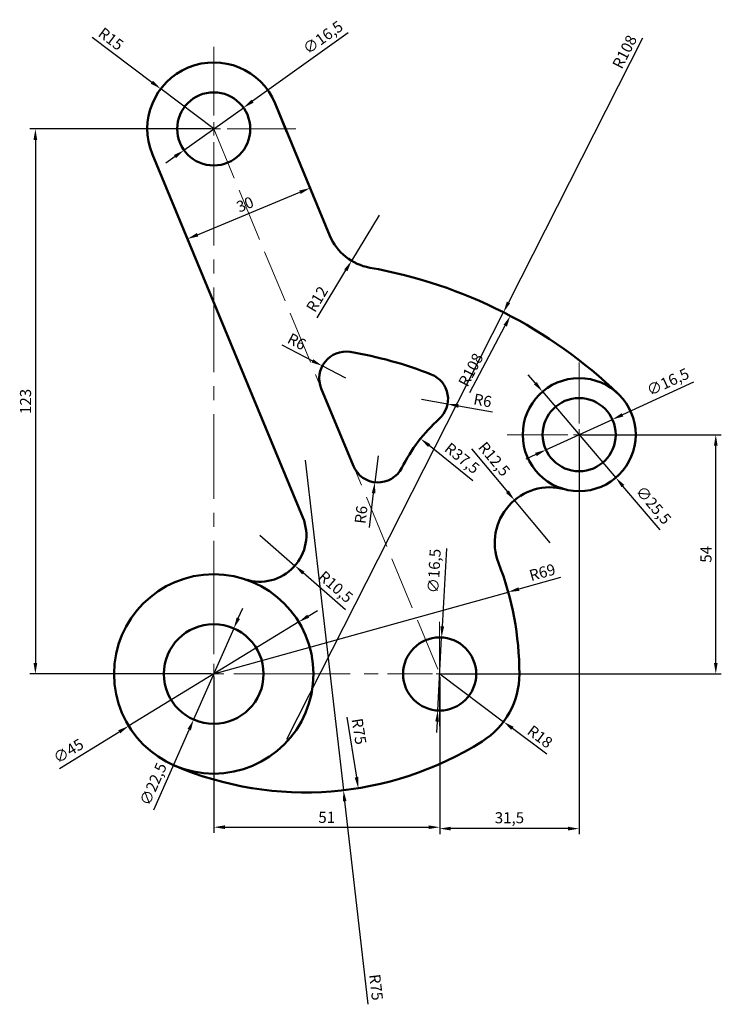
# Model space of a CAD drawing. Units: millimetres. Extents: x 2645 to 2804, y 1499 to 1721.
import ezdxf

# ---------------------------------------------------------------- set-up
doc = ezdxf.new("R2010")
doc.units = ezdxf.units.MM
doc.linetypes.add('ACAD_ISO02W100', pattern=[15, 12, -3])
doc.linetypes.add('CENTER2', pattern=[28.575, 19.05, -3.175, 3.175, -3.175])
for name, color, linetype, lineweight in [('M-CNTR', 4, 'CENTER2', 18), ('M-CONS', 8, 'ACAD_ISO02W100', 18), ('M-DIMS', 2, 'Continuous', 25), ('M-OUTL', 7, 'Continuous', 50)]:
    doc.layers.add(name, color=color, linetype=linetype, lineweight=lineweight)
doc.styles.get("Standard").update_dxf_attribs({"font": 'arial.ttf'})
doc.dimstyles.new('ISO-25', dxfattribs={"dimtxt": 2.5, "dimasz": 2.5, "dimexe": 1.25, "dimexo": 0.625, "dimtad": 1, "dimtxsty": 'Standard', "dimcen": 2.5, "dimadec": 0, "dimazin": 0, "dimtfac": 1, "dimtmove": 0, "dimatfit": 3, "dimfxl": 1, "dimarcsym": 0})

# ---------------------------------------------------------------- blocks, each defined once
blk = doc.blocks.new('*U1')
at = {"layer": 'M-CNTR', "color": 0, "transparency": 16777216}
for p, q in [((0, 4.5), (0, 26)), ((-26, 0), (-4.5, 0)), ((4.5, 0), (26, 0)), ((0, -26), (0, -4.5))]:
    blk.add_line(p, q, dxfattribs=at)
at = {"layer": 'M-CNTR', "color": 0, "linetype": 'Continuous', "transparency": 16777216}
for p, q in [((0, -2.25), (0, 2.25)), ((-2.25, 0), (2.25, 0))]:
    blk.add_line(p, q, dxfattribs=at)
blk = doc.blocks.new('*U2')
at = {"layer": 'M-CNTR', "color": 0, "transparency": 16777216}
for p, q in [((0, 2.55), (0, 16.25)), ((-16.25, 0), (-2.55, 0)), ((2.55, 0), (16.25, 0)), ((0, -16.25), (0, -2.55))]:
    blk.add_line(p, q, dxfattribs=at)
at = {"layer": 'M-CNTR', "color": 0, "linetype": 'Continuous', "transparency": 16777216}
for p, q in [((-1.275, 0), (1.275, 0)), ((0, -1.275), (0, 1.275))]:
    blk.add_line(p, q, dxfattribs=at)
blk = doc.blocks.new('*U3')
at = {"layer": 'M-CNTR', "color": 0, "transparency": 16777216}
for p, q in [((0, 3), (0, 18.5)), ((-18.5, 0), (-3, 0)), ((3, 0), (18.5, 0)), ((0, -18.5), (0, -3))]:
    blk.add_line(p, q, dxfattribs=at)
at = {"layer": 'M-CNTR', "color": 0, "linetype": 'Continuous', "transparency": 16777216}
for p, q in [((-1.5, 0), (1.5, 0)), ((0, -1.5), (0, 1.5))]:
    blk.add_line(p, q, dxfattribs=at)
blk = doc.blocks.new('*U4')
at = {"layer": 'M-CNTR', "color": 0, "transparency": 16777216}
for p, q in [((0, 1.65), (0, 11.75)), ((-11.75, 0), (-1.65, 0)), ((1.65, 0), (11.75, 0)), ((0, -11.75), (0, -1.65))]:
    blk.add_line(p, q, dxfattribs=at)
at = {"layer": 'M-CNTR', "color": 0, "linetype": 'Continuous', "transparency": 16777216}
for p, q in [((-0.825, 0), (0.825, 0)), ((0, -0.825), (0, 0.825))]:
    blk.add_line(p, q, dxfattribs=at)
blk = doc.blocks.new('*U5')
at = {"layer": 'M-CNTR', "color": 0, "transparency": 16777216}
blk.add_line((0, 52), (0, -52), dxfattribs=at)
blk = doc.blocks.new('*U6')
at = {"layer": 'M-CNTR', "color": 0, "transparency": 16777216}
blk.add_line((-18.025, 0), (18.025, 0), dxfattribs=at)
blk = doc.blocks.new('*D7')
at = {"layer": 'Defpoints', "color": 0, "transparency": 16777216}
for p in [(2689.12, 1696.37), (2648.85, 1573.37), (2689.12, 1573.37)]:
    blk.add_point(p, dxfattribs=at)
at = {"layer": 'M-DIMS', "color": 0, "lineweight": -2, "transparency": 16777216}
for p, q in [((2688.49, 1696.37), (2647.6, 1696.37)), ((2648.85, 1693.87), (2648.85, 1575.87)), ((2688.49, 1573.37), (2647.6, 1573.37))]:
    blk.add_line(p, q, dxfattribs=at)
at = {"layer": 'M-DIMS', "color": 0, "transparency": 16777216}
for points in [[(2648.43, 1693.87), (2649.27, 1693.87), (2648.85, 1696.37)], [(2648.43, 1575.87), (2649.27, 1575.87), (2648.85, 1573.37)]]:
    blk.add_solid(points, dxfattribs=at)
at = {"layer": 'M-DIMS', "color": 0, "transparency": 16777216, "insert": (2646.95, 1634.87), "char_height": 2.5, "attachment_point": 5, "rotation": 90}
blk.add_mtext('123', dxfattribs=at)
blk = doc.blocks.new('*D8')
at = {"layer": 'Defpoints', "color": 0, "transparency": 16777216}
for p in [(2689.12, 1573.37), (2740.12, 1573.37), (2740.12, 1538.79)]:
    blk.add_point(p, dxfattribs=at)
at = {"layer": 'M-DIMS', "color": 0, "lineweight": -2, "transparency": 16777216}
for p, q in [((2689.12, 1572.75), (2689.12, 1537.54)), ((2740.12, 1572.75), (2740.12, 1537.54)), ((2691.62, 1538.79), (2737.62, 1538.79))]:
    blk.add_line(p, q, dxfattribs=at)
at = {"layer": 'M-DIMS', "color": 0, "transparency": 16777216}
for points in [[(2691.62, 1539.21), (2691.62, 1538.38), (2689.12, 1538.79)], [(2737.62, 1539.21), (2737.62, 1538.38), (2740.12, 1538.79)]]:
    blk.add_solid(points, dxfattribs=at)
at = {"layer": 'M-DIMS', "color": 0, "transparency": 16777216, "insert": (2714.62, 1540.69), "char_height": 2.5, "attachment_point": 5}
blk.add_mtext('51', dxfattribs=at)
blk = doc.blocks.new('*D9')
at = {"layer": 'Defpoints', "color": 0, "transparency": 16777216}
for p in [(2771.62, 1627.37), (2740.12, 1572.81), (2740.12, 1538.47)]:
    blk.add_point(p, dxfattribs=at)
at = {"layer": 'M-DIMS', "color": 0, "lineweight": -2, "transparency": 16777216}
for p, q in [((2771.62, 1626.75), (2771.62, 1537.22)), ((2740.12, 1572.19), (2740.12, 1537.22)), ((2769.12, 1538.47), (2742.62, 1538.47))]:
    blk.add_line(p, q, dxfattribs=at)
at = {"layer": 'M-DIMS', "color": 0, "transparency": 16777216}
for points in [[(2742.62, 1538.89), (2742.62, 1538.06), (2740.12, 1538.47)], [(2769.12, 1538.89), (2769.12, 1538.06), (2771.62, 1538.47)]]:
    blk.add_solid(points, dxfattribs=at)
at = {"layer": 'M-DIMS', "color": 0, "transparency": 16777216, "insert": (2755.87, 1540.6), "char_height": 2.5, "attachment_point": 5}
blk.add_mtext('31,5', dxfattribs=at)
blk = doc.blocks.new('*D10')
at = {"layer": 'Defpoints', "color": 0, "transparency": 16777216}
for p in [(2771.62, 1627.37), (2802.45, 1627.37), (2740.12, 1573.37)]:
    blk.add_point(p, dxfattribs=at)
at = {"layer": 'M-DIMS', "color": 0, "lineweight": -2, "transparency": 16777216}
for p, q in [((2772.24, 1627.37), (2803.7, 1627.37)), ((2802.45, 1575.87), (2802.45, 1624.87)), ((2740.74, 1573.37), (2803.7, 1573.37))]:
    blk.add_line(p, q, dxfattribs=at)
at = {"layer": 'M-DIMS', "color": 0, "transparency": 16777216}
for points in [[(2802.03, 1624.87), (2802.87, 1624.87), (2802.45, 1627.37)], [(2802.03, 1575.87), (2802.87, 1575.87), (2802.45, 1573.37)]]:
    blk.add_solid(points, dxfattribs=at)
at = {"layer": 'M-DIMS', "color": 0, "transparency": 16777216, "insert": (2800.56, 1600.37), "char_height": 2.5, "attachment_point": 5, "rotation": 90}
blk.add_mtext('54', dxfattribs=at)
blk = doc.blocks.new('*D11')
at = {"layer": 'Defpoints', "color": 0, "transparency": 16777216}
for p in [(2708.31, 1585.11), (2669.92, 1561.63)]:
    blk.add_point(p, dxfattribs=at)
at = {"layer": 'M-DIMS', "color": 0, "lineweight": -2, "transparency": 16777216}
for p, q in [((2710.44, 1586.42), (2712.57, 1587.72)), ((2708.31, 1585.11), (2669.92, 1561.63)), ((2654.28, 1552.06), (2667.79, 1560.33))]:
    blk.add_line(p, q, dxfattribs=at)
at = {"layer": 'M-DIMS', "color": 0, "transparency": 16777216}
for points in [[(2710.22, 1586.77), (2710.66, 1586.06), (2708.31, 1585.11)], [(2667.57, 1560.68), (2668.01, 1559.97), (2669.92, 1561.63)]]:
    blk.add_solid(points, dxfattribs=at)
at = {"layer": 'M-DIMS', "color": 0, "transparency": 16777216, "insert": (2656.48, 1555.72), "char_height": 2.5, "attachment_point": 5, "rotation": 31.4542}
blk.add_mtext('∅45', dxfattribs=at)
blk = doc.blocks.new('*D12')
at = {"layer": 'Defpoints', "color": 0, "transparency": 16777216}
for p in [(2693.65, 1583.66), (2684.58, 1563.08)]:
    blk.add_point(p, dxfattribs=at)
at = {"layer": 'M-DIMS', "color": 0, "lineweight": -2, "transparency": 16777216}
for p, q in [((2694.66, 1585.95), (2695.67, 1588.24)), ((2693.65, 1583.66), (2684.58, 1563.08)), ((2675.6, 1542.71), (2683.57, 1560.79))]:
    blk.add_line(p, q, dxfattribs=at)
at = {"layer": 'M-DIMS', "color": 0, "transparency": 16777216}
for points in [[(2694.28, 1586.12), (2695.04, 1585.78), (2693.65, 1583.66)], [(2683.19, 1560.96), (2683.95, 1560.62), (2684.58, 1563.08)]]:
    blk.add_solid(points, dxfattribs=at)
at = {"layer": 'M-DIMS', "color": 0, "transparency": 16777216, "insert": (2675.73, 1548.39), "char_height": 2.5, "attachment_point": 5, "rotation": 66.2096}
blk.add_mtext('∅22,5', dxfattribs=at)
blk = doc.blocks.new('*D13')
at = {"layer": 'Defpoints', "color": 0, "transparency": 16777216}
for p in [(2763.35, 1637.08), (2779.88, 1617.66)]:
    blk.add_point(p, dxfattribs=at)
at = {"layer": 'M-DIMS', "color": 0, "lineweight": -2, "transparency": 16777216}
for p, q in [((2761.73, 1638.98), (2760.11, 1640.88)), ((2763.35, 1637.08), (2779.88, 1617.66)), ((2789.92, 1605.88), (2781.5, 1615.76))]:
    blk.add_line(p, q, dxfattribs=at)
at = {"layer": 'M-DIMS', "color": 0, "transparency": 16777216}
for points in [[(2762.04, 1639.25), (2761.41, 1638.71), (2763.35, 1637.08)], [(2781.82, 1616.03), (2781.19, 1615.49), (2779.88, 1617.66)]]:
    blk.add_solid(points, dxfattribs=at)
at = {"layer": 'M-DIMS', "color": 0, "transparency": 16777216, "insert": (2788.17, 1611.27), "char_height": 2.5, "attachment_point": 5, "rotation": 310.4214}
blk.add_mtext('∅25,5', dxfattribs=at)
blk = doc.blocks.new('*D14')
at = {"layer": 'Defpoints', "color": 0, "transparency": 16777216}
for p in [(2695.83, 1701.16), (2682.4, 1691.58)]:
    blk.add_point(p, dxfattribs=at)
at = {"layer": 'M-DIMS', "color": 0, "lineweight": -2, "transparency": 16777216}
for p, q in [((2719.47, 1718.04), (2697.86, 1702.62)), ((2682.4, 1691.58), (2695.83, 1701.16)), ((2680.37, 1690.12), (2678.33, 1688.67))]:
    blk.add_line(p, q, dxfattribs=at)
at = {"layer": 'M-DIMS', "color": 0, "transparency": 16777216}
for points in [[(2697.62, 1702.96), (2698.11, 1702.28), (2695.83, 1701.16)], [(2680.12, 1690.46), (2680.61, 1689.79), (2682.4, 1691.58)]]:
    blk.add_solid(points, dxfattribs=at)
at = {"layer": 'M-DIMS', "color": 0, "transparency": 16777216, "insert": (2713.95, 1716.76), "char_height": 2.5, "attachment_point": 5, "rotation": 35.5241}
blk.add_mtext('∅16,5', dxfattribs=at)
blk = doc.blocks.new('*D15')
at = {"layer": 'Defpoints', "color": 0, "transparency": 16777216}
for p in [(2779.12, 1630.81), (2764.11, 1623.94)]:
    blk.add_point(p, dxfattribs=at)
at = {"layer": 'M-DIMS', "color": 0, "lineweight": -2, "transparency": 16777216}
for p, q in [((2797.44, 1639.2), (2781.39, 1631.85)), ((2764.11, 1623.94), (2779.12, 1630.81)), ((2761.84, 1622.89), (2759.57, 1621.85))]:
    blk.add_line(p, q, dxfattribs=at)
at = {"layer": 'M-DIMS', "color": 0, "transparency": 16777216}
for points in [[(2781.22, 1632.23), (2781.56, 1631.47), (2779.12, 1630.81)], [(2761.67, 1623.27), (2762.02, 1622.52), (2764.11, 1623.94)]]:
    blk.add_solid(points, dxfattribs=at)
at = {"layer": 'M-DIMS', "color": 0, "transparency": 16777216, "insert": (2791.77, 1638.99), "char_height": 2.5, "attachment_point": 5, "rotation": 24.6069}
blk.add_mtext('∅16,5', dxfattribs=at)
blk = doc.blocks.new('*D16')
at = {"layer": 'Defpoints', "color": 0, "transparency": 16777216}
for p in [(2740.56, 1581.61), (2739.67, 1565.13)]:
    blk.add_point(p, dxfattribs=at)
at = {"layer": 'M-DIMS', "color": 0, "lineweight": -2, "transparency": 16777216}
for p, q in [((2741.64, 1601.71), (2740.69, 1584.11)), ((2739.67, 1565.13), (2740.56, 1581.61)), ((2739.54, 1562.64), (2739.41, 1560.14))]:
    blk.add_line(p, q, dxfattribs=at)
at = {"layer": 'M-DIMS', "color": 0, "transparency": 16777216}
for points in [[(2740.28, 1584.13), (2741.11, 1584.08), (2740.56, 1581.61)], [(2739.12, 1562.66), (2739.96, 1562.61), (2739.67, 1565.13)]]:
    blk.add_solid(points, dxfattribs=at)
at = {"layer": 'M-DIMS', "color": 0, "transparency": 16777216, "insert": (2739.19, 1596.59), "char_height": 2.5, "attachment_point": 5, "rotation": 86.9302}
blk.add_mtext('∅16,5', dxfattribs=at)
blk = doc.blocks.new('*D17')
at = {"layer": 'Defpoints', "color": 0, "transparency": 16777216}
for p in [(2677.14, 1705.41), (2689.12, 1696.37)]:
    blk.add_point(p, dxfattribs=at)
at = {"layer": 'M-DIMS', "color": 0, "lineweight": -2, "transparency": 16777216}
for p, q in [((2661.68, 1717.08), (2675.15, 1706.91)), ((2689.12, 1696.37), (2677.14, 1705.41))]:
    blk.add_line(p, q, dxfattribs=at)
at = {"layer": 'M-DIMS', "color": 0, "transparency": 16777216}
blk.add_solid([(2675.4, 1707.25), (2674.9, 1706.58), (2677.14, 1705.41)], dxfattribs=at)
at = {"layer": 'M-DIMS', "color": 0, "transparency": 16777216, "insert": (2665.72, 1716.42), "char_height": 2.5, "attachment_point": 5, "rotation": 322.951}
blk.add_mtext('R15', dxfattribs=at)
blk = doc.blocks.new('*D18')
at = {"layer": 'Defpoints', "color": 0, "transparency": 16777216}
for p in [(2726.43, 1676.87), (2720.23, 1666.6)]:
    blk.add_point(p, dxfattribs=at)
at = {"layer": 'M-DIMS', "color": 0, "lineweight": -2, "transparency": 16777216}
for p, q in [((2726.43, 1676.87), (2720.23, 1666.6)), ((2712.46, 1653.73), (2718.94, 1664.46))]:
    blk.add_line(p, q, dxfattribs=at)
at = {"layer": 'M-DIMS', "color": 0, "transparency": 16777216}
blk.add_solid([(2718.58, 1664.67), (2719.29, 1664.24), (2720.23, 1666.6)], dxfattribs=at)
at = {"layer": 'M-DIMS', "color": 0, "transparency": 16777216, "insert": (2712.71, 1657.79), "char_height": 2.5, "attachment_point": 5, "rotation": 58.8826}
blk.add_mtext('R12', dxfattribs=at)
blk = doc.blocks.new('*D19')
at = {"layer": 'Defpoints', "color": 0, "transparency": 16777216}
for p in [(2756.08, 1654.18), (2705.62, 1558.69)]:
    blk.add_point(p, dxfattribs=at)
at = {"layer": 'M-DIMS', "color": 0, "lineweight": -2, "transparency": 16777216}
blk.add_line((2746.95, 1636.91), (2754.91, 1651.97), dxfattribs=at)
at = {"layer": 'M-DIMS', "color": 0, "transparency": 16777216}
blk.add_solid([(2754.54, 1652.16), (2755.28, 1651.77), (2756.08, 1654.18)], dxfattribs=at)
at = {"layer": 'M-DIMS', "color": 0, "transparency": 16777216, "insert": (2747.42, 1641.85), "char_height": 2.5, "attachment_point": 5, "rotation": 62.146}
blk.add_mtext('R108', dxfattribs=at)
blk = doc.blocks.new('*D20')
at = {"layer": 'Defpoints', "color": 0, "transparency": 16777216}
for p in [(2757.02, 1612.58), (2765.04, 1602.99)]:
    blk.add_point(p, dxfattribs=at)
at = {"layer": 'M-DIMS', "color": 0, "lineweight": -2, "transparency": 16777216}
for p, q in [((2747.29, 1624.2), (2755.41, 1614.49)), ((2765.04, 1602.99), (2757.02, 1612.58))]:
    blk.add_line(p, q, dxfattribs=at)
at = {"layer": 'M-DIMS', "color": 0, "transparency": 16777216}
blk.add_solid([(2755.73, 1614.76), (2755.09, 1614.22), (2757.02, 1612.58)], dxfattribs=at)
at = {"layer": 'M-DIMS', "color": 0, "transparency": 16777216, "insert": (2752.18, 1621.67), "char_height": 2.5, "attachment_point": 5, "rotation": 309.937}
blk.add_mtext('R12,5', dxfattribs=at)
blk = doc.blocks.new('*D21')
at = {"layer": 'Defpoints', "color": 0, "transparency": 16777216}
for p in [(2735.8, 1626.47), (2765.04, 1602.99)]:
    blk.add_point(p, dxfattribs=at)
at = {"layer": 'M-DIMS', "color": 0, "lineweight": -2, "transparency": 16777216}
blk.add_line((2747.62, 1616.98), (2737.75, 1624.9), dxfattribs=at)
at = {"layer": 'M-DIMS', "color": 0, "transparency": 16777216}
blk.add_solid([(2738.01, 1625.23), (2737.49, 1624.58), (2735.8, 1626.47)], dxfattribs=at)
at = {"layer": 'M-DIMS', "color": 0, "transparency": 16777216, "insert": (2744.99, 1621.82), "char_height": 2.5, "attachment_point": 5, "rotation": 321.2426}
blk.add_mtext('R37,5', dxfattribs=at)
blk = doc.blocks.new('*D22')
at = {"layer": 'Defpoints', "color": 0, "transparency": 16777216}
for p in [(2713.62, 1642.88), (2718.94, 1640.11)]:
    blk.add_point(p, dxfattribs=at)
at = {"layer": 'M-DIMS', "color": 0, "lineweight": -2, "transparency": 16777216}
for p, q in [((2704.5, 1647.62), (2711.4, 1644.03)), ((2718.94, 1640.11), (2713.62, 1642.88))]:
    blk.add_line(p, q, dxfattribs=at)
at = {"layer": 'M-DIMS', "color": 0, "transparency": 16777216}
blk.add_solid([(2711.59, 1644.4), (2711.21, 1643.66), (2713.62, 1642.88)], dxfattribs=at)
at = {"layer": 'M-DIMS', "color": 0, "transparency": 16777216, "insert": (2707.72, 1648.09), "char_height": 2.5, "attachment_point": 5, "rotation": 332.5021}
blk.add_mtext('R6', dxfattribs=at)
blk = doc.blocks.new('*D23')
at = {"layer": 'Defpoints', "color": 0, "transparency": 16777216}
for p in [(2736.01, 1635.39), (2741.91, 1634.3)]:
    blk.add_point(p, dxfattribs=at)
at = {"layer": 'M-DIMS', "color": 0, "lineweight": -2, "transparency": 16777216}
for p, q in [((2736.01, 1635.39), (2741.91, 1634.3)), ((2752.02, 1632.43), (2744.37, 1633.84))]:
    blk.add_line(p, q, dxfattribs=at)
at = {"layer": 'M-DIMS', "color": 0, "transparency": 16777216}
blk.add_solid([(2744.45, 1634.25), (2744.3, 1633.43), (2741.91, 1634.3)], dxfattribs=at)
at = {"layer": 'M-DIMS', "color": 0, "transparency": 16777216, "insert": (2749.77, 1634.78), "char_height": 2.5, "attachment_point": 5, "rotation": 349.5394}
blk.add_mtext('R6', dxfattribs=at)
blk = doc.blocks.new('*D24')
at = {"layer": 'Defpoints', "color": 0, "transparency": 16777216}
for p in [(2726.21, 1622.58), (2725.49, 1616.63)]:
    blk.add_point(p, dxfattribs=at)
at = {"layer": 'M-DIMS', "color": 0, "lineweight": -2, "transparency": 16777216}
for p, q in [((2726.21, 1622.58), (2725.49, 1616.63)), ((2724.26, 1606.42), (2725.19, 1614.15))]:
    blk.add_line(p, q, dxfattribs=at)
at = {"layer": 'M-DIMS', "color": 0, "transparency": 16777216}
blk.add_solid([(2724.78, 1614.2), (2725.6, 1614.1), (2725.49, 1616.63)], dxfattribs=at)
at = {"layer": 'M-DIMS', "color": 0, "transparency": 16777216, "insert": (2722.69, 1609.27), "char_height": 2.5, "attachment_point": 5, "rotation": 83.1412}
blk.add_mtext('R6', dxfattribs=at)
blk = doc.blocks.new('*D25')
at = {"layer": 'Defpoints', "color": 0, "transparency": 16777216}
for p in [(2709.78, 1621.63), (2721.74, 1547.59)]:
    blk.add_point(p, dxfattribs=at)
at = {"layer": 'M-DIMS', "color": 0, "lineweight": -2, "transparency": 16777216}
blk.add_line((2719.15, 1563.63), (2721.34, 1550.06), dxfattribs=at)
at = {"layer": 'M-DIMS', "color": 0, "transparency": 16777216}
blk.add_solid([(2721.75, 1550.12), (2720.93, 1549.99), (2721.74, 1547.59)], dxfattribs=at)
at = {"layer": 'M-DIMS', "color": 0, "transparency": 16777216, "insert": (2721.6, 1560.36), "char_height": 2.5, "attachment_point": 5, "rotation": 279.1695}
blk.add_mtext('R75', dxfattribs=at)
blk = doc.blocks.new('*D26')
at = {"layer": 'Defpoints', "color": 0, "transparency": 16777216}
for p in [(2699.53, 1604.69), (2707.45, 1597.8)]:
    blk.add_point(p, dxfattribs=at)
at = {"layer": 'M-DIMS', "color": 0, "lineweight": -2, "transparency": 16777216}
for p, q in [((2699.53, 1604.69), (2707.45, 1597.8)), ((2718.89, 1587.85), (2709.34, 1596.16))]:
    blk.add_line(p, q, dxfattribs=at)
at = {"layer": 'M-DIMS', "color": 0, "transparency": 16777216}
blk.add_solid([(2709.61, 1596.47), (2709.06, 1595.84), (2707.45, 1597.8)], dxfattribs=at)
at = {"layer": 'M-DIMS', "color": 0, "transparency": 16777216, "insert": (2716.45, 1592.79), "char_height": 2.5, "attachment_point": 5, "rotation": 319.0015}
blk.add_mtext('R10,5', dxfattribs=at)
blk = doc.blocks.new('*D27')
at = {"layer": 'Defpoints', "color": 0, "transparency": 16777216}
for p in [(2755.59, 1591.86), (2689.12, 1573.37)]:
    blk.add_point(p, dxfattribs=at)
at = {"layer": 'M-DIMS', "color": 0, "lineweight": -2, "transparency": 16777216}
for p, q in [((2767.37, 1595.14), (2758, 1592.53)), ((2689.12, 1573.37), (2755.59, 1591.86))]:
    blk.add_line(p, q, dxfattribs=at)
at = {"layer": 'M-DIMS', "color": 0, "transparency": 16777216}
blk.add_solid([(2757.89, 1592.93), (2758.11, 1592.13), (2755.59, 1591.86)], dxfattribs=at)
at = {"layer": 'M-DIMS', "color": 0, "transparency": 16777216, "insert": (2763.38, 1596), "char_height": 2.5, "attachment_point": 5, "rotation": 15.5436}
blk.add_mtext('R69', dxfattribs=at)
blk = doc.blocks.new('*D28')
at = {"layer": 'Defpoints', "color": 0, "transparency": 16777216}
for p in [(2740.12, 1573.37), (2754.54, 1562.6)]:
    blk.add_point(p, dxfattribs=at)
at = {"layer": 'M-DIMS', "color": 0, "lineweight": -2, "transparency": 16777216}
for p, q in [((2740.12, 1573.37), (2754.54, 1562.6)), ((2764.34, 1555.28), (2756.54, 1561.1))]:
    blk.add_line(p, q, dxfattribs=at)
at = {"layer": 'M-DIMS', "color": 0, "transparency": 16777216}
blk.add_solid([(2756.79, 1561.44), (2756.29, 1560.77), (2754.54, 1562.6)], dxfattribs=at)
at = {"layer": 'M-DIMS', "color": 0, "transparency": 16777216, "insert": (2762.58, 1558.97), "char_height": 2.5, "attachment_point": 5, "rotation": 323.2484}
blk.add_mtext('R18', dxfattribs=at)
blk = doc.blocks.new('*D29')
at = {"layer": 'Defpoints', "color": 0, "transparency": 16777216}
for p in [(2710.89, 1683.03), (2711.13, 1682.43), (2683.42, 1670.94)]:
    blk.add_point(p, dxfattribs=at)
at = {"layer": 'M-DIMS', "color": 0, "lineweight": -2, "transparency": 16777216}
for p, q in [((2710.89, 1683.01), (2710.41, 1684.19)), ((2685.48, 1672.5), (2708.58, 1682.07)), ((2683.18, 1671.52), (2682.69, 1672.69))]:
    blk.add_line(p, q, dxfattribs=at)
at = {"layer": 'M-DIMS', "color": 0, "transparency": 16777216}
for points in [[(2708.42, 1682.46), (2708.74, 1681.69), (2710.89, 1683.03)], [(2685.32, 1672.88), (2685.64, 1672.11), (2683.17, 1671.54)]]:
    blk.add_solid(points, dxfattribs=at)
at = {"layer": 'M-DIMS', "color": 0, "transparency": 16777216, "insert": (2696.3, 1679.04), "char_height": 2.5, "attachment_point": 5, "rotation": 22.5206}
blk.add_mtext('30', dxfattribs=at)
blk = doc.blocks.new('*D30')
at = {"layer": 'Defpoints', "color": 0, "transparency": 16777216}
for p in [(2754.52, 1654.98), (2705.62, 1558.69)]:
    blk.add_point(p, dxfattribs=at)
at = {"layer": 'M-DIMS', "color": 0, "lineweight": -2, "transparency": 16777216}
for p, q in [((2785.94, 1716.85), (2755.65, 1657.21)), ((2705.62, 1558.69), (2754.52, 1654.98))]:
    blk.add_line(p, q, dxfattribs=at)
at = {"layer": 'M-DIMS', "color": 0, "transparency": 16777216}
blk.add_solid([(2755.28, 1657.4), (2756.02, 1657.02), (2754.52, 1654.98)], dxfattribs=at)
at = {"layer": 'M-DIMS', "color": 0, "transparency": 16777216, "insert": (2782.16, 1713.62), "char_height": 2.5, "attachment_point": 5, "rotation": 63.0782}
blk.add_mtext('R108', dxfattribs=at)
blk = doc.blocks.new('*D31')
at = {"layer": 'Defpoints', "color": 0, "transparency": 16777216}
for p in [(2709.78, 1621.63), (2718.4, 1547.13)]:
    blk.add_point(p, dxfattribs=at)
at = {"layer": 'M-DIMS', "color": 0, "lineweight": -2, "transparency": 16777216}
for p, q in [((2709.78, 1621.63), (2718.4, 1547.13)), ((2723.98, 1498.83), (2718.69, 1544.64))]:
    blk.add_line(p, q, dxfattribs=at)
at = {"layer": 'M-DIMS', "color": 0, "transparency": 16777216}
blk.add_solid([(2719.1, 1544.69), (2718.27, 1544.6), (2718.4, 1547.13)], dxfattribs=at)
at = {"layer": 'M-DIMS', "color": 0, "transparency": 16777216, "insert": (2725.45, 1502.64), "char_height": 2.5, "attachment_point": 5, "rotation": 276.5954}
blk.add_mtext('R75', dxfattribs=at)

msp = doc.modelspace()

# ---------------------------------------------------------------- linework, layer by layer
at = {"layer": 'M-CONS'}
msp.add_line((2689.116, 1696.371), (2740.116, 1573.371), dxfattribs=at)
at = {"layer": 'M-OUTL'}
for p, q in [((2702.972, 1702.116), (2715.345, 1672.274)), ((2702.972, 1702.116), (2705.653, 1695.65)), ((2705.653, 1695.65), (2705.844, 1695.188)), ((2675.26, 1690.625), (2709.226, 1608.707)), ((2720.663, 1620.287), (2713.398, 1637.808))]:
    msp.add_line(p, q, dxfattribs=at)
for centre, radius in [((2689.116, 1696.371), 8.25), ((2771.616, 1627.371), 12.75), ((2771.616, 1627.371), 8.25), ((2689.116, 1573.371), 22.5), ((2689.116, 1573.371), 11.25), ((2740.116, 1573.371), 8.25)]:
    msp.add_circle(centre, radius, dxfattribs=at)
for centre, radius, start, end in [((2689.116, 1696.371), 15, 22.52057, 202.52057), ((2726.43, 1676.871), 12, 202.52057, 260.01375), ((2705.621, 1558.689), 108, 46.1429, 80.01375), ((2718.94, 1640.106), 6, 80.70901, 202.52057), ((2705.621, 1558.689), 88.5, 68.38426, 80.70901), ((2736.012, 1635.387), 6, 311.86424, 68.38426), ((2765.042, 1602.991), 37.5, 131.86424, 153.22879), ((2726.205, 1622.585), 6, 202.52057, 333.22879), ((2765.042, 1602.991), 12.5, 74.91052, 201.3118), ((2699.526, 1604.685), 10.5, 251.61046, 22.52057), ((2689.116, 1573.371), 69, 0, 21.3118), ((2740.116, 1573.371), 18, 302.14886, 0), ((2709.785, 1621.631), 75, 246.81524, 302.14886)]:
    msp.add_arc(centre, radius, start, end, dxfattribs=at)

# ---------------------------------------------------------------- block references
at = {"layer": 'M-CNTR'}
for name, p in [('*U3', (2689.116, 1696.371)), ('*U5', (2689.116, 1637.121)), ('*U2', (2771.616, 1627.371)), ('*U1', (2689.116, 1573.371)), ('*U4', (2740.116, 1573.371)), ('*U6', (2718.891, 1573.371))]:
    msp.add_blockref(name, p, dxfattribs=at)

# ---------------------------------------------------------------- dimensions: what is measured, and where the dimension line sits
at = {"layer": 'M-DIMS'}
for p1, p2, picture, middle in [((2682.401, 1691.577), (2695.83, 1701.164), '*D14', (2715.206, 1714.997)), ((2764.115, 1623.935), (2779.116, 1630.806), '*D15', (2792.674, 1637.015)), ((2739.674, 1565.132), (2740.558, 1581.609), '*D16', (2741.355, 1596.472)), ((2708.309, 1585.111), (2669.922, 1561.63), '*D11', (2657.505, 1554.034)), ((2693.654, 1583.665), (2684.578, 1563.077), '*D12', (2677.715, 1547.511))]:
    dim = msp.add_diameter_dim_2p(p1=p1, p2=p2, dimstyle='ISO-25', override={"dimclrd": 0, "dimclre": 0, "dimclrt": 0}, dxfattribs=at)
    dim.commit()
    dim.dimension.update_dxf_attribs({"geometry": picture, "text_midpoint": middle, "dimtype": 163})
for center, mpoint, override, picture, middle in [((2689.116, 1696.371), (2677.144, 1705.408), {"dimclrd": 0, "dimclre": 0, "dimclrt": 0}, '*D17', (2664.572, 1714.899)), ((2705.621, 1558.689), (2754.52, 1654.984), {"dimdec": 0, "dimlfac": 1, "dimrnd": 0, "dimzin": 0, "dimdsep": 46, "dimlunit": 2}, '*D30', (2783.86, 1712.762)), ((2726.43, 1676.871), (2720.228, 1666.597), {"dimclrd": 0, "dimclre": 0, "dimclrt": 0}, '*D18', (2714.323, 1656.814)), ((2705.621, 1558.689), (2756.08, 1654.176), {"dimclrd": 0, "dimclre": 0, "dimclrt": 0}, '*D19', (2749.097, 1640.961)), ((2765.042, 1602.991), (2735.8, 1626.467), {"dimclrd": 0, "dimclre": 0, "dimclrt": 0}, '*D21', (2743.658, 1620.158)), ((2709.785, 1621.631), (2721.736, 1547.589), {"dimclrd": 0, "dimclre": 0, "dimclrt": 0}, '*D25', (2719.724, 1560.058)), ((2709.785, 1621.631), (2718.399, 1547.127), {"dimdec": 0, "dimlfac": 1, "dimrnd": 0, "dimzin": 0, "dimdsep": 46, "dimlunit": 2}, '*D31', (2723.568, 1502.425))]:
    dim = msp.add_radius_dim(center=center, mpoint=mpoint, dimstyle='ISO-25', override=override, dxfattribs=at)
    dim.commit()
    dim.dimension.update_dxf_attribs({"geometry": picture, "text_midpoint": middle, "dimtype": 164})
for base, p1, p2, picture, middle in [((2648.849, 1573.371), (2689.116, 1696.371), (2689.116, 1573.371), '*D7', (2646.946, 1634.871)), ((2802.452, 1627.371), (2740.116, 1573.371), (2771.616, 1627.371), '*D10', (2800.555, 1600.371))]:
    dim = msp.add_linear_dim(base=base, p1=p1, p2=p2, angle=90, dimstyle='ISO-25', override={"dimclrd": 0, "dimclre": 0, "dimclrt": 0}, dxfattribs=at)
    dim.commit()
    dim.dimension.update_dxf_attribs({"geometry": picture, "text_midpoint": middle})
dim = msp.add_aligned_dim(p1=(2683.42, 1670.944), p2=(2711.132, 1682.434), distance=0.645, dimstyle='ISO-25', override={"dimclrd": 0, "dimclre": 0, "dimclrt": 0}, dxfattribs=at)
dim.commit()
dim.dimension.update_dxf_attribs({"geometry": '*D29', "text_midpoint": (2696.301, 1679.042)})
for center, mpoint, picture, middle in [((2718.94, 1640.106), (2713.618, 1642.877), '*D22', (2707.719, 1648.091)), ((2736.012, 1635.387), (2741.912, 1634.298), '*D23', (2749.77, 1634.78)), ((2765.042, 1602.991), (2757.018, 1612.576), '*D20', (2752.18, 1621.668)), ((2726.205, 1622.585), (2725.489, 1616.628), '*D24', (2722.688, 1609.27)), ((2699.526, 1604.685), (2707.451, 1597.797), '*D26', (2716.453, 1592.791)), ((2689.116, 1573.371), (2755.592, 1591.861), '*D27', (2763.382, 1596.001)), ((2740.116, 1573.371), (2754.538, 1562.6), '*D28', (2762.578, 1558.969))]:
    dim = msp.add_radius_dim(center=center, mpoint=mpoint, dimstyle='ISO-25', override={"dimclrd": 0, "dimclre": 0, "dimclrt": 0}, dxfattribs=at)
    dim.commit()
    dim.dimension.update_dxf_attribs({"geometry": picture, "text_midpoint": middle})
dim = msp.add_diameter_dim_2p(p1=(2763.349, 1637.077), p2=(2779.883, 1617.664), dimstyle='ISO-25', override={"dimclrd": 0, "dimclre": 0, "dimclrt": 0}, dxfattribs=at)
dim.commit()
dim.dimension.update_dxf_attribs({"geometry": '*D13', "text_midpoint": (2788.174, 1611.273)})
for base, p1, p2, picture, middle in [((2740.116, 1538.473), (2771.616, 1627.371), (2740.116, 1572.811), '*D9', (2755.866, 1540.6)), ((2740.116, 1538.792), (2689.116, 1573.371), (2740.116, 1573.371), '*D8', (2714.616, 1540.693))]:
    dim = msp.add_linear_dim(base=base, p1=p1, p2=p2, dimstyle='ISO-25', override={"dimclrd": 0, "dimclre": 0, "dimclrt": 0}, dxfattribs=at)
    dim.commit()
    dim.dimension.update_dxf_attribs({"geometry": picture, "text_midpoint": middle})

doc.saveas('drawing.dxf')
